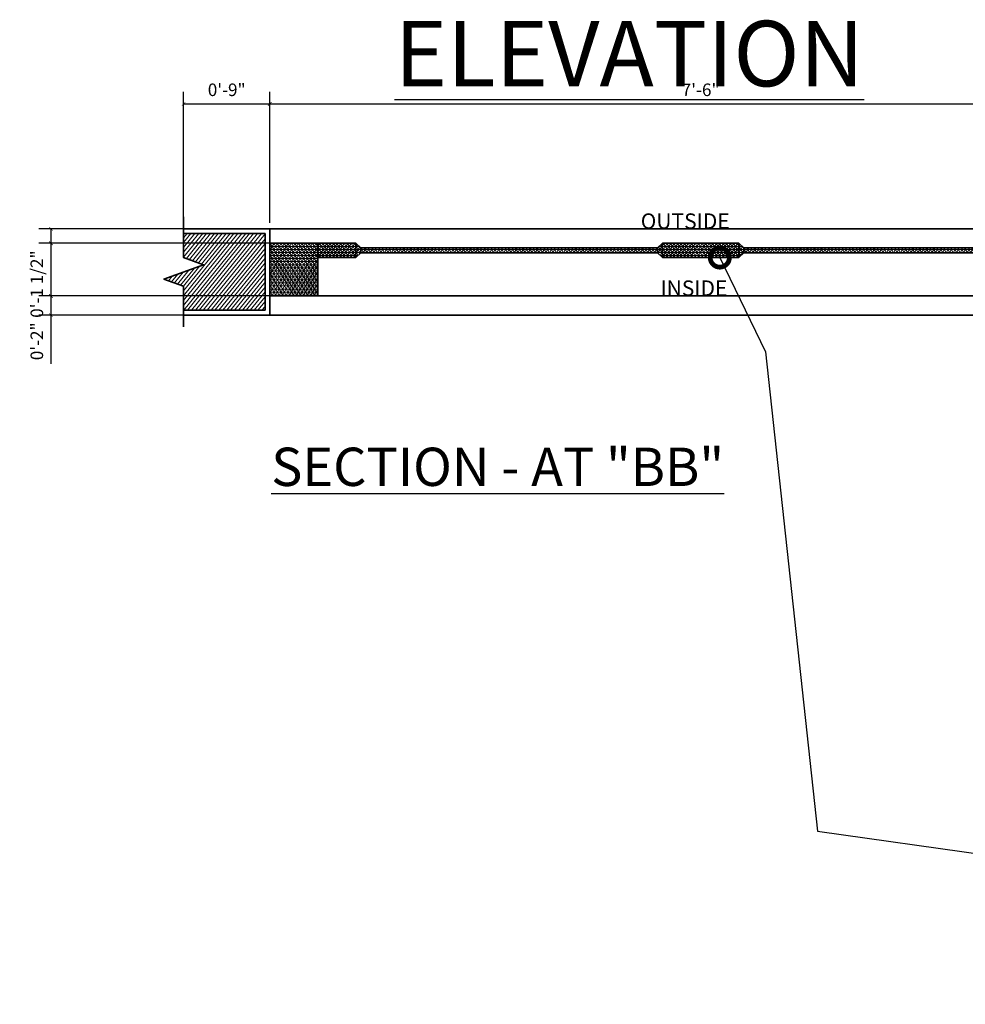
# Model space of a CAD drawing. Units: inches. Extents: x 1926 to 2169, y 1541 to 1783.
# Tile 1 of 3: x 1926 to 2025, y 1541 to 1644. Entities that reach past the tile are written whole.
import ezdxf
from ezdxf import colors
from ezdxf.entities.mleader import LeaderData, LeaderLine
from ezdxf.math import Vec2, Vec3

# ---------------------------------------------------------------- set-up
doc = ezdxf.new("R2010")
doc.units = ezdxf.units.IN
for name, color, linetype, lineweight in [('A-ANNO-DIMS', 2, 'Continuous', 18), ('A-ANNO-TEXT', 3, 'Continuous', 25), ('A-DETL', 7, 'Continuous', 35), ('A-DETL-PATT', 8, 'Continuous', 18)]:
    doc.layers.add(name, color=color, linetype=linetype, lineweight=lineweight)
doc.styles.get("Standard").update_dxf_attribs({"font": 'arial.ttf'})
doc.dimstyles.new('ISO-25', dxfattribs={"dimtxt": 1.3125, "dimasz": 0.375, "dimexe": 1.25, "dimexo": 0.625, "dimtad": 1, "dimzin": 3, "dimlunit": 4, "dimtxsty": 'Standard', "dimblk": 'ARCHTICK', "dimcen": 0.09, "dimadec": 0, "dimazin": 0, "dimtfac": 1, "dimtofl": 0, "dimtmove": 0, "dimatfit": 3, "dimfxl": 1, "dimarcsym": 0})

# ---------------------------------------------------------------- blocks, each defined once
blk = doc.blocks.new('_DotSmall')
at = {"color": 0, "linetype": 'ByBlock', "const_width": 0.5}
blk.add_lwpolyline([(-0.0625, 0, 1), (0.0625, 0, 1)], format="xyb", close=True, dxfattribs=at)
blk = doc.blocks.new('_ArchTick')
at = {"color": 0, "linetype": 'ByBlock', "const_width": 0.15}
blk.add_lwpolyline([(-0.5, -0.5), (0.5, 0.5)], dxfattribs=at)
blk = doc.blocks.new('*D39')
at = {"layer": 'A-ANNO-DIMS', "color": 0, "lineweight": -2, "transparency": 16777216}
for p, q in [((1943.54, 1622.67), (1943.54, 1636.34)), ((1952.54, 1622.67), (1952.54, 1636.34)), ((1943.54, 1635.09), (1952.54, 1635.09))]:
    blk.add_line(p, q, dxfattribs=at)
at = {"layer": 'DEFPOINTS', "color": 0, "transparency": 16777216}
for p in [(1952.54, 1635.09), (1943.54, 1622.04), (1952.54, 1622.04)]:
    blk.add_point(p, dxfattribs=at)
at = {"layer": 'A-ANNO-DIMS', "color": 0, "lineweight": -2, "transparency": 16777216, "xscale": 0.375, "yscale": 0.375, "zscale": 0.375, "rotation": 180}
blk.add_blockref('_ArchTick', (1943.54, 1635.09), dxfattribs=at)
at = {"layer": 'A-ANNO-DIMS', "color": 0, "lineweight": -2, "transparency": 16777216, "xscale": 0.375, "yscale": 0.375, "zscale": 0.375}
blk.add_blockref('_ArchTick', (1952.54, 1635.09), dxfattribs=at)
at = {"layer": 'A-ANNO-DIMS', "color": 0, "transparency": 16777216, "insert": (1948.04, 1636.39), "char_height": 1.312, "attachment_point": 5}
blk.add_mtext('0\'-9"', dxfattribs=at)
blk = doc.blocks.new('*D40')
at = {"layer": 'A-ANNO-DIMS', "color": 0, "lineweight": -2, "transparency": 16777216}
for p, q in [((1952.54, 1622.67), (1952.54, 1636.34)), ((2042.54, 1622.67), (2042.54, 1636.34)), ((1952.54, 1635.09), (2042.54, 1635.09))]:
    blk.add_line(p, q, dxfattribs=at)
at = {"layer": 'DEFPOINTS', "color": 0, "transparency": 16777216}
for p in [(2042.54, 1635.09), (1952.54, 1622.04), (2042.54, 1622.04)]:
    blk.add_point(p, dxfattribs=at)
at = {"layer": 'A-ANNO-DIMS', "color": 0, "lineweight": -2, "transparency": 16777216, "xscale": 0.375, "yscale": 0.375, "zscale": 0.375, "rotation": 180}
blk.add_blockref('_ArchTick', (1952.54, 1635.09), dxfattribs=at)
at = {"layer": 'A-ANNO-DIMS', "color": 0, "lineweight": -2, "transparency": 16777216, "xscale": 0.375, "yscale": 0.375, "zscale": 0.375}
blk.add_blockref('_ArchTick', (2042.54, 1635.09), dxfattribs=at)
at = {"layer": 'A-ANNO-DIMS', "color": 0, "transparency": 16777216, "insert": (1997.54, 1636.39), "char_height": 1.312, "attachment_point": 5}
blk.add_mtext('7\'-6"', dxfattribs=at)
blk = doc.blocks.new('*D42')
at = {"layer": 'A-ANNO-DIMS', "color": 0, "lineweight": -2, "transparency": 16777216}
for p, q in [((1951.92, 1622.04), (1928.43, 1622.04)), ((1929.68, 1622.04), (1929.68, 1620.54)), ((1956.92, 1620.54), (1928.43, 1620.54)), ((1929.68, 1620.54), (1929.68, 1612.37))]:
    blk.add_line(p, q, dxfattribs=at)
at = {"layer": 'DEFPOINTS', "color": 0, "transparency": 16777216}
for p in [(1952.54, 1622.04), (1929.68, 1620.54), (1957.54, 1620.54)]:
    blk.add_point(p, dxfattribs=at)
at = {"layer": 'A-ANNO-DIMS', "color": 0, "lineweight": -2, "transparency": 16777216, "xscale": 0.375, "yscale": 0.375, "zscale": 0.375}
for p, rotation in [((1929.68, 1622.04), 90), ((1929.68, 1620.54), 270)]:
    blk.add_blockref('_ArchTick', p, dxfattribs=dict(at, rotation=rotation))
at = {"layer": 'A-ANNO-DIMS', "color": 0, "transparency": 16777216, "insert": (1928.38, 1616.27), "char_height": 1.312, "attachment_point": 5, "rotation": 90}
blk.add_mtext('0\'-1 1/2"', dxfattribs=at)
blk = doc.blocks.new('*D43')
at = {"layer": 'A-ANNO-DIMS', "color": 0, "lineweight": -2, "transparency": 16777216}
for p, q in [((1956.92, 1615.04), (1928.43, 1615.04)), ((1929.68, 1615.04), (1929.68, 1613.04)), ((1951.92, 1613.04), (1928.43, 1613.04)), ((1929.68, 1613.04), (1929.68, 1607.93))]:
    blk.add_line(p, q, dxfattribs=at)
at = {"layer": 'DEFPOINTS', "color": 0, "transparency": 16777216}
for p in [(1957.54, 1615.04), (1929.68, 1613.04), (1952.54, 1613.04)]:
    blk.add_point(p, dxfattribs=at)
at = {"layer": 'A-ANNO-DIMS', "color": 0, "lineweight": -2, "transparency": 16777216, "xscale": 0.375, "yscale": 0.375, "zscale": 0.375}
for p, rotation in [((1929.68, 1615.04), 90), ((1929.68, 1613.04), 270)]:
    blk.add_blockref('_ArchTick', p, dxfattribs=dict(at, rotation=rotation))
at = {"layer": 'A-ANNO-DIMS', "color": 0, "transparency": 16777216, "insert": (1928.38, 1610.3), "char_height": 1.312, "attachment_point": 5, "rotation": 90}
blk.add_mtext('0\'-2"', dxfattribs=at)

msp = doc.modelspace()

# ---------------------------------------------------------------- hatches: boundary and pattern name
at = {"layer": 'A-DETL-PATT'}
h = msp.add_hatch(dxfattribs=at)
h.set_pattern_fill('ANSI31', color=256, scale=0.1, angle=186)
h.paths.add_polyline_path([(1952.04, 1621.543), (1943.54, 1621.543), (1943.54, 1619.043), (1945.601, 1618.293), (1941.48, 1616.793), (1943.54, 1616.043), (1943.54, 1613.543), (1952.04, 1613.543)])
h = msp.add_hatch(dxfattribs=at)
h.set_pattern_fill('NET3', color=256, scale=0.1)
h.paths.add_polyline_path([(1993.54, 1620.543), (1997.54, 1620.543), (1997.54, 1619.043), (1993.54, 1619.043)])
h.paths.add_polyline_path([(1986.8, 1620.043), (1993.04, 1620.043), (1993.04, 1619.543), (1986.8, 1619.543)])
h.paths.add_polyline_path([(1993.04, 1620.043), (1993.54, 1620.543), (1993.54, 1619.043), (1993.04, 1619.543)])
h.paths.add_polyline_path([(1962.04, 1620.043), (1986.3, 1620.043), (1986.3, 1619.543), (1962.04, 1619.543)])
h.paths.add_polyline_path([(1957.54, 1620.543), (1961.54, 1620.543), (1961.54, 1619.043), (1957.54, 1619.043)])
h.paths.add_polyline_path([(1961.54, 1620.543), (1962.04, 1620.043), (1962.04, 1619.543), (1961.54, 1619.043)])
h.paths.add_polyline_path([(1952.54, 1620.543), (1957.54, 1620.543), (1957.54, 1615.043), (1952.54, 1615.043)])
h.paths.add_polyline_path([(1986.3, 1620.043), (1986.8, 1620.043), (1986.8, 1619.543), (1986.3, 1619.543)])
h = msp.add_hatch(dxfattribs=at)
h.set_pattern_fill('NET3', color=256, scale=0.1)
h.paths.add_polyline_path([(2001.54, 1620.543), (1997.54, 1620.543), (1997.54, 1619.043), (2001.54, 1619.043)])
h.paths.add_polyline_path([(2008.28, 1620.043), (2002.04, 1620.043), (2002.04, 1619.543), (2008.28, 1619.543)])
h.paths.add_polyline_path([(2002.04, 1620.043), (2001.54, 1620.543), (2001.54, 1619.043), (2002.04, 1619.543)])
h.paths.add_polyline_path([(2033.04, 1620.043), (2008.78, 1620.043), (2008.78, 1619.543), (2033.04, 1619.543)])
h.paths.add_polyline_path([(2037.54, 1620.543), (2033.54, 1620.543), (2033.54, 1619.043), (2037.54, 1619.043)])
h.paths.add_polyline_path([(2033.54, 1620.543), (2033.04, 1620.043), (2033.04, 1619.543), (2033.54, 1619.043)])
h.paths.add_polyline_path([(2042.54, 1620.543), (2037.54, 1620.543), (2037.54, 1615.043), (2042.54, 1615.043)])
h.paths.add_polyline_path([(2008.78, 1620.043), (2008.28, 1620.043), (2008.28, 1619.543), (2008.78, 1619.543)])

# ---------------------------------------------------------------- linework, layer by layer
at = {"layer": 'A-DETL'}
for p, q in [((2003.8, 1622.043), (1943.54, 1622.043)), ((1952.04, 1621.543), (1943.54, 1621.543)), ((1952.04, 1613.543), (1952.04, 1621.543)), ((1952.54, 1613.043), (1952.54, 1622.043)), ((1991.28, 1622.043), (2051.54, 1622.043)), ((1957.54, 1620.543), (1952.54, 1620.543)), ((1957.54, 1615.043), (1957.54, 1620.543)), ((1957.54, 1620.543), (1961.54, 1620.543)), ((1961.54, 1619.043), (1961.54, 1620.543)), ((1962.04, 1620.043), (1961.54, 1620.543)), ((1993.04, 1620.043), (1993.54, 1620.543)), ((1993.54, 1619.043), (1993.54, 1620.543)), ((1997.54, 1620.543), (1993.54, 1620.543)), ((1997.54, 1620.543), (2001.54, 1620.543)), ((2001.54, 1619.043), (2001.54, 1620.543)), ((2002.04, 1620.043), (2001.54, 1620.543)), ((1961.54, 1619.043), (1962.04, 1619.543)), ((1962.04, 1619.543), (1962.04, 1620.043)), ((1962.04, 1620.043), (1993.04, 1620.043)), ((1962.04, 1619.543), (1993.04, 1619.543)), ((1993.04, 1619.543), (1993.04, 1620.043)), ((1993.54, 1619.043), (1993.04, 1619.543)), ((2001.54, 1619.043), (2002.04, 1619.543)), ((2033.04, 1620.043), (2002.04, 1620.043)), ((2002.04, 1619.543), (2002.04, 1620.043)), ((2033.04, 1619.543), (2002.04, 1619.543)), ((1957.54, 1619.043), (1961.54, 1619.043)), ((1997.54, 1619.043), (1993.54, 1619.043)), ((1997.54, 1619.043), (2001.54, 1619.043)), ((1957.54, 1615.043), (1952.54, 1615.043)), ((1957.54, 1615.043), (2037.54, 1615.043)), ((1952.04, 1613.543), (1943.54, 1613.543)), ((1995.78, 1613.043), (1943.54, 1613.043)), ((1991.28, 1613.043), (2051.54, 1613.043))]:
    msp.add_line(p, q, dxfattribs=at)
msp.add_lwpolyline([(1943.54, 1611.793), (1943.54, 1616.043), (1941.48, 1616.793), (1945.601, 1618.293), (1943.54, 1619.043), (1943.54, 1623.293)], dxfattribs=at)

# ---------------------------------------------------------------- texts
at = {"layer": 'A-ANNO-TEXT'}
for s, p in [('OUTSIDE', (1991.28, 1622.043)), ('INSIDE', (1993.339, 1615.043))]:
    msp.add_text(s, height=1.6109, dxfattribs=at).set_placement(p)
at = {"layer": 'A-ANNO-TEXT', "attachment_point": 1}
for s, width, insert, char_height in [('{\\LELEVATION}', 60.21423, (1965.572, 1643.76), 6.83314), ('{\\LSECTION - AT "BB"}', 57.58278, (1952.692, 1599.191), 4)]:
    msp.add_mtext_dynamic_manual_height_columns(s, width=width, gutter_width=34.166, heights=[0], dxfattribs=dict(at, insert=insert, char_height=char_height))

# ---------------------------------------------------------------- dimensions: what is measured, and where the dimension line sits
at = {"layer": 'A-ANNO-DIMS'}
for base, p1, p2, picture, middle in [((1952.54, 1635.093), (1943.54, 1622.043), (1952.54, 1622.043), '*D39', (1948.04, 1636.388)), ((2042.54, 1635.093), (1952.54, 1622.043), (2042.54, 1622.043), '*D40', (1997.54, 1636.388))]:
    dim = msp.add_linear_dim(base=base, p1=p1, p2=p2, dimstyle='ISO-25', override={"dimdec": 1, "dimlfac": 1, "dimrnd": 0, "dimzin": 1, "dimdsep": 46, "dimlunit": 4, "dimfrac": 2}, dxfattribs=at)
    dim.commit()
    dim.dimension.update_dxf_attribs({"geometry": picture, "text_midpoint": middle})
for base, p1, p2, picture, middle in [((1929.68, 1620.543), (1952.54, 1622.043), (1957.54, 1620.543), '*D42', (1928.376, 1616.269)), ((1929.68, 1613.043), (1957.54, 1615.043), (1952.54, 1613.043), '*D43', (1928.384, 1610.299))]:
    dim = msp.add_linear_dim(base=base, p1=p1, p2=p2, angle=90, dimstyle='ISO-25', override={"dimdec": 1, "dimlfac": 1, "dimrnd": 0, "dimzin": 1, "dimdsep": 46, "dimlunit": 4, "dimfrac": 2}, dxfattribs=at)
    dim.commit()
    dim.dimension.update_dxf_attribs({"geometry": picture, "text_midpoint": middle})

# ---------------------------------------------------------------- leaders
at = {"layer": 'A-ANNO-TEXT'}
ml = msp.add_multileader_mtext('Standard', dxfattribs=at)
ml.set_content('\\A1;MIDDLE STYLE 1 {\\H0.7x;\\S1/2;}"X4"THICK', color=256)
ml.set_leader_properties()
ml.set_arrow_properties(name='DOTSMALL')
ml.build(insert=Vec2(0, 0))
ctx = ml.context
ctx.base_point, ctx.char_height, ctx.plane_origin = Vec3(2063.638, 1552.694), 2, Vec3(1999.54, 1619.043)
notes = []
notes.append((ctx, [(0, (1, 1, 0), (2055.638, 1552.694), (1, 0), 8, [(0, [(1999.54, 1619.043), (2004.296, 1609.195), (2009.741, 1559.148)], 0, [])])]))
ctx.mtext.insert, ctx.mtext.flow_direction = Vec3(2065.638, 1553.711), 5
for ctx, leaders in notes:
    for number, flags, end, landing, length, lines in leaders:
        leader = LeaderData()
        leader.index, (leader.has_last_leader_line, leader.has_dogleg_vector, leader.attachment_direction) = number, flags
        leader.last_leader_point, leader.dogleg_vector, leader.dogleg_length = Vec3(end), Vec3(landing), length
        for number, points, colour, breaks in lines:
            line = LeaderLine()
            line.index, line.vertices, line.color, line.breaks = number, Vec3.list(points), colors.encode_raw_color(colour), breaks
            leader.lines.append(line)
        ctx.leaders.append(leader)

doc.saveas('drawing.dxf')
